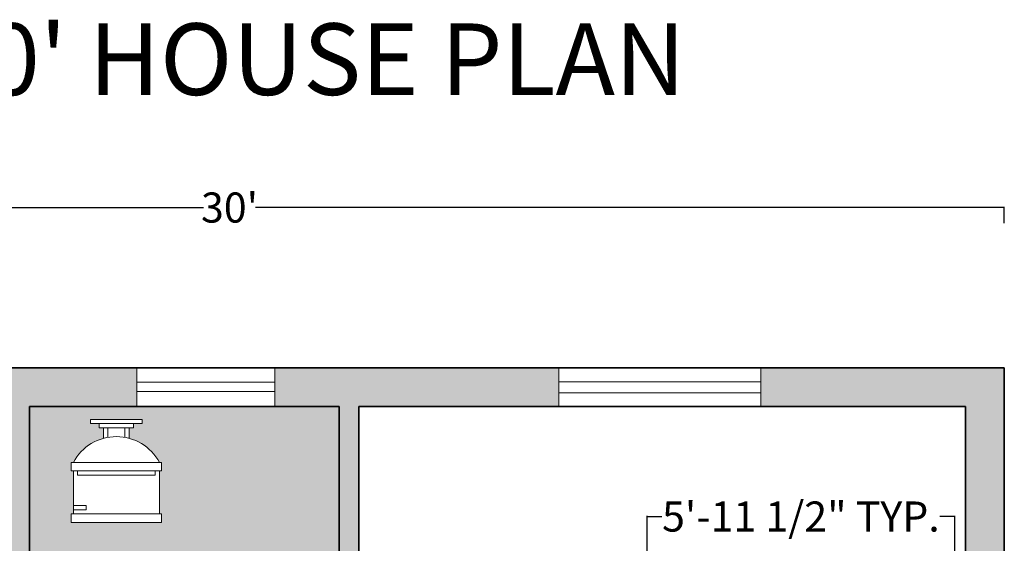
# Model space of a CAD drawing. Units: inches. Extents: x 2167 to 2589, y 1680 to 2489.
# Tile 38 of 38: x 2346 to 2575, y 2367 to 2489. Entities that reach past the tile are written whole.
import ezdxf

# ---------------------------------------------------------------- set-up
doc = ezdxf.new("R2010")
doc.units = ezdxf.units.IN
doc.header["$MEASUREMENT"] = 0
doc.layers.get('0').update_dxf_attribs({"color": 250})
for name, color, linetype, lineweight in [('A-ANNO-DIMS', 2, 'Continuous', 18), ('A-FLOR-FIXT', 8, 'Continuous', 18), ('A-FLOR-TILE-PATT', 252, 'Continuous', 13), ('A-WALL-PATT', 250, 'Continuous', 13), ('C-PROP', 7, 'Continuous', 35), ('text', 7, 'Continuous', 25), ('walls', 7, 'Continuous', 35), ('windows', 141, 'Continuous', 18)]:
    doc.layers.add(name, color=color, linetype=linetype, lineweight=lineweight)
doc.styles.get("Standard").update_dxf_attribs({"font": 'arial.ttf'})
doc.dimstyles.get("Standard").update_dxf_attribs({"dimtxt": 7, "dimasz": 0.18, "dimexe": 0.18, "dimexo": 0.0625, "dimgap": 0.09, "dimtad": 0, "dimtih": 1, "dimtoh": 1, "dimdec": 1, "dimzin": 0, "dimdsep": 46, "dimlunit": 3, "dimtxsty": 'Standard', "dimcen": 0.09, "dimadec": 0, "dimazin": 0, "dimtfac": 1, "dimtdec": 1, "dimtofl": 0, "dimtmove": 0, "dimatfit": 3, "dimfxl": 1, "dimtolj": 1, "dimtzin": 0, "dimarcsym": 0})

# ---------------------------------------------------------------- blocks, each defined once
blk = doc.blocks.new('*U11')
for p, q in [((-10, 22), (-10, 12)), ((-10, 21), (-7, 21)), ((-7, 21), (-7, 20)), ((10, 12), (10, 22)), ((-7, 20), (-10, 20)), ((10.5, 12), (-10.5, 12)), ((-10.5, 10), (-10.5, 12)), ((9, 13), (-9, 13)), ((-9, 13), (-9, 12)), ((9, 12), (9, 13)), ((10.5, 12), (10.5, 10)), ((10.5, 10), (-10.5, 10)), ((-3, 4.4065), (-3, 2)), ((-2, 2), (-2, 4.1658)), ((2, 4.1658), (2, 2)), ((3, 2), (3, 4.4065)), ((4, 2), (-4, 2)), ((-4, 2), (-4, 1)), ((4, 1), (4, 2))]:
    blk.add_line(p, q)
for points in [[(10.5, 22), (10.5, 24), (-10.5, 24), (-10.5, 22)], [(6, 0), (6, 1), (-6, 1), (-6, 0)]]:
    blk.add_lwpolyline(points, close=True)
blk.add_arc((0, 15.3333), 11.3333, 208.0725, 331.9275)
blk = doc.blocks.new('*D23')
at = {"layer": 'A-ANNO-DIMS', "color": 0, "lineweight": -2, "transparency": 16777216}
for p, q in [((2215.05, 2441.31), (2215.05, 2445.11)), ((2215.23, 2444.93), (2389.02, 2444.93)), ((2574.87, 2444.93), (2401.08, 2444.93)), ((2575.05, 2441.31), (2575.05, 2445.11))]:
    blk.add_line(p, q, dxfattribs=at)
at = {"layer": 'A-ANNO-DIMS', "color": 0, "transparency": 16777216}
for points in [[(2215.23, 2444.96), (2215.23, 2444.9), (2215.05, 2444.93)], [(2574.87, 2444.96), (2574.87, 2444.9), (2575.05, 2444.93)]]:
    blk.add_solid(points, dxfattribs=at)
at = {"layer": 'Defpoints', "color": 0, "transparency": 16777216}
for p in [(2575.05, 2444.93), (2215.05, 2441.25), (2575.05, 2441.25)]:
    blk.add_point(p, dxfattribs=at)
at = {"layer": 'A-ANNO-DIMS', "color": 0, "transparency": 16777216, "insert": (2395.05, 2444.93), "char_height": 7, "attachment_point": 5}
blk.add_mtext("\\A1;30'", dxfattribs=at)
blk = doc.blocks.new('*D44')
at = {"layer": 'A-ANNO-DIMS', "color": 0, "lineweight": -2, "transparency": 16777216}
for p, q in [((2492.05, 2361.43), (2492.05, 2373.28)), ((2492.23, 2373.1), (2495.49, 2373.1)), ((2563.35, 2373.1), (2560.09, 2373.1)), ((2563.53, 2361.43), (2563.53, 2373.28))]:
    blk.add_line(p, q, dxfattribs=at)
at = {"layer": 'A-ANNO-DIMS', "color": 0, "transparency": 16777216}
for points in [[(2492.23, 2373.13), (2492.23, 2373.07), (2492.05, 2373.1)], [(2563.35, 2373.13), (2563.35, 2373.07), (2563.53, 2373.1)]]:
    blk.add_solid(points, dxfattribs=at)
at = {"layer": 'Defpoints', "color": 0, "transparency": 16777216}
for p in [(2492.05, 2373.1), (2492.05, 2361.37), (2563.53, 2361.37)]:
    blk.add_point(p, dxfattribs=at)
at = {"layer": 'A-ANNO-DIMS', "color": 0, "transparency": 16777216, "insert": (2527.79, 2373.1), "char_height": 7, "attachment_point": 5}
blk.add_mtext('\\A1;5\'-11 1/2" TYP.', dxfattribs=at)

msp = doc.modelspace()

# ---------------------------------------------------------------- hatches: boundary and pattern name
at = {"layer": 'A-FLOR-TILE-PATT'}
h = msp.add_hatch(dxfattribs=at)
h.set_pattern_fill('ANGLE', color=256, scale=5)
h.set_pattern_definition([(0, (0, 0), (0, 1.375), [1, -0.375]), (90, (0, 0), (-1.375, 1e-16), [1, -0.375])])
h.paths.add_polyline_path([(2420.55, 2398.69), (2348.55, 2398.69), (2348.55, 2314.69), (2420.55, 2314.69), (2420.55, 2326.49), (2398.64, 2326.49), (2398.64, 2327.5), (2398.66, 2327.5, -0.388161), (2420.55, 2349.43)])
h.paths.add_polyline_path([(2379.26, 2371.69), (2358.26, 2371.69), (2358.26, 2373.69), (2358.76, 2373.69), (2358.76, 2383.69), (2358.26, 2383.69), (2358.26, 2385.69), (2358.76, 2385.69, -0.206081), (2365.76, 2391.29), (2365.76, 2393.69), (2364.76, 2393.69), (2364.76, 2394.69), (2362.76, 2394.69), (2362.76, 2395.69), (2374.76, 2395.69), (2374.76, 2394.69), (2372.76, 2394.69), (2372.76, 2393.69), (2371.76, 2393.69), (2371.76, 2391.29, -0.206081), (2378.76, 2385.69), (2379.26, 2385.69), (2379.26, 2383.69), (2378.76, 2383.69), (2378.76, 2373.69), (2379.26, 2373.69)], flags=16)
edge = h.paths.add_edge_path(flags=16)
edge.add_ellipse((2357.9, 2328.17), major_axis=(0.02, -7.48), ratio=0.576535, start_angle=272.6137, end_angle=620.1108, ccw=False)
edge.add_ellipse((2357.9, 2328.17), major_axis=(0.02, -7.48), ratio=0.576535, start_angle=260.1108, end_angle=272.6137, ccw=False)
h.paths.add_polyline_path([(2359.92, 2328.19, -1), (2356.35, 2328.19, -1)], flags=0)
h.paths.add_polyline_path([(2356.71, 2328.19, -1), (2359.56, 2328.19, -1)], flags=0)
h.paths.add_polyline_path([(2355.42, 2328.91), (2355.42, 2327.96), (2354.63, 2327.96), (2354.63, 2329.51), (2354.92, 2329.51), (2354.92, 2328.91)], flags=0)
at = {"layer": 'A-WALL-PATT'}
h = msp.add_hatch(color=256, dxfattribs=at)
h.dxf.hatch_style = 1
h.paths.add_polyline_path([(2471.54, 2407.69), (2405.59, 2407.69), (2405.59, 2398.69), (2420.55, 2398.69), (2420.55, 2349.43, -0.011499), (2421.6, 2349.45), (2425.05, 2349.45), (2425.05, 2398.69), (2471.54, 2398.69)])
h.paths.add_polyline_path([(2420.55, 2250.19), (2348.55, 2250.19), (2348.55, 2310.19), (2420.55, 2310.19)], flags=16)
h.paths.add_polyline_path([(2320.06, 2212.92, -0.014764), (2320.1, 2214.19), (2224.05, 2214.19), (2224.05, 2346.19), (2250.86, 2346.19), (2250.86, 2350.69), (2224.05, 2350.69), (2224.05, 2398.69), (2250.76, 2398.69), (2250.76, 2407.69), (2215.05, 2407.69), (2215.05, 2179.66), (2218.49, 2179.66), (2224.05, 2179.66), (2224.05, 2209.69), (2314.05, 2209.69), (2314.05, 2202.4), (2314.78, 2202.4), (2318.55, 2202.4), (2318.55, 2209.69), (2320.06, 2209.69)])
h.paths.add_polyline_path([(2310.92, 2349.42, -0.014764), (2310.96, 2350.69), (2297.23, 2350.69), (2297.23, 2346.19), (2310.92, 2346.19)], flags=17)
h.paths.add_polyline_path([(2425.05, 2275.27), (2420.55, 2275.27), (2420.55, 2292.87), (2425.05, 2292.87), (2425.05, 2326.49), (2421.6, 2326.49), (2420.55, 2326.49), (2420.55, 2314.69), (2348.55, 2314.69), (2348.55, 2398.69), (2373.55, 2398.69), (2373.55, 2404.36), (2373.55, 2407.69), (2297.68, 2407.69), (2297.68, 2398.69), (2344.05, 2398.69), (2344.05, 2350.69), (2332.45, 2350.69), (2332.45, 2349.42), (2332.45, 2346.19), (2344.05, 2346.19), (2344.05, 2214.19), (2341.59, 2214.19), (2341.59, 2212.92), (2341.59, 2209.69), (2348.55, 2209.69), (2348.55, 2245.69), (2425.05, 2245.69)])
h = msp.add_hatch(color=256, dxfattribs=at)
h.dxf.hatch_style = 1
h.paths.add_polyline_path([(2575.05, 2407.69), (2518.45, 2407.69), (2518.45, 2398.69), (2566.05, 2398.69), (2566.05, 2210.05), (2568.65, 2210.05), (2575.05, 2210.05)])
h.paths.add_polyline_path([(2503.01, 2166.19), (2497.84, 2166.19, -0.014764), (2497.88, 2164.92), (2497.88, 2161.69), (2503.01, 2161.69)])

# ---------------------------------------------------------------- linework, layer by layer
at = {"layer": 'C-PROP'}
for p, q in [((2215.05, 2407.69), (2575.05, 2407.69)), ((2575.05, 2407.69), (2575.05, 1687.69))]:
    msp.add_line(p, q, dxfattribs=at)
at = {"layer": 'walls'}
for p, q in [((2348.55, 2314.69), (2348.55, 2398.69)), ((2348.55, 2398.69), (2420.55, 2398.69)), ((2420.55, 2349.43), (2420.55, 2398.69)), ((2425.05, 2230.69), (2425.05, 2398.69)), ((2425.05, 2398.69), (2566.05, 2398.69)), ((2566.05, 2398.69), (2566.05, 2166.19))]:
    msp.add_line(p, q, dxfattribs=at)
at = {"layer": 'windows'}
for p, q in [((2373.55, 2398.69), (2373.55, 2407.69)), ((2373.55, 2407.69), (2405.59, 2407.69)), ((2405.59, 2407.69), (2405.59, 2398.69)), ((2471.54, 2407.69), (2471.54, 2398.69)), ((2518.45, 2407.69), (2471.54, 2407.69)), ((2518.45, 2398.69), (2518.45, 2407.69)), ((2373.55, 2398.69), (2373.55, 2404.36)), ((2373.55, 2404.36), (2405.59, 2404.36)), ((2405.59, 2404.36), (2405.59, 2402.14)), ((2471.54, 2404.42), (2518.45, 2404.42)), ((2518.45, 2404.42), (2518.45, 2401.88)), ((2405.59, 2402.14), (2373.55, 2402.14)), ((2518.45, 2401.88), (2471.54, 2401.88)), ((2405.59, 2398.69), (2373.55, 2398.69)), ((2471.54, 2398.69), (2518.45, 2398.69))]:
    msp.add_line(p, q, dxfattribs=at)

# ---------------------------------------------------------------- block references
at = {"layer": 'A-FLOR-FIXT', "xscale": -1, "rotation": 180}
msp.add_blockref('*U11', (2368.76, 2395.69), dxfattribs=at)

# ---------------------------------------------------------------- texts
at = {"layer": 'text'}
msp.add_text("30' X 60' HOUSE PLAN", height=16.6398, dxfattribs=at).set_placement((2271.09, 2471.1))

# ---------------------------------------------------------------- dimensions: what is measured, and where the dimension line sits
at = {"layer": 'A-ANNO-DIMS'}
dim = msp.add_linear_dim(base=(2575.05, 2444.93), p1=(2215.05, 2441.25), p2=(2575.05, 2441.25), dimstyle='Standard', override={"dimclrd": 0, "dimclre": 0, "dimclrt": 0}, dxfattribs=at)
dim.commit()
dim.dimension.update_dxf_attribs({"geometry": '*D23', "text_midpoint": (2395.05, 2444.93)})
dim = msp.add_linear_dim(base=(2492.05, 2373.1), p1=(2563.53, 2361.37), p2=(2492.05, 2361.37), angle=180, text='<> TYP.', dimstyle='Standard', override={"dimdec": 1, "dimlfac": 1, "dimrnd": 0, "dimzin": 1, "dimdsep": 46, "dimlunit": 4, "dimfrac": 2}, dxfattribs=at)
dim.commit()
dim.dimension.update_dxf_attribs({"geometry": '*D44', "text_midpoint": (2527.79, 2373.1)})

doc.saveas('drawing.dxf')
